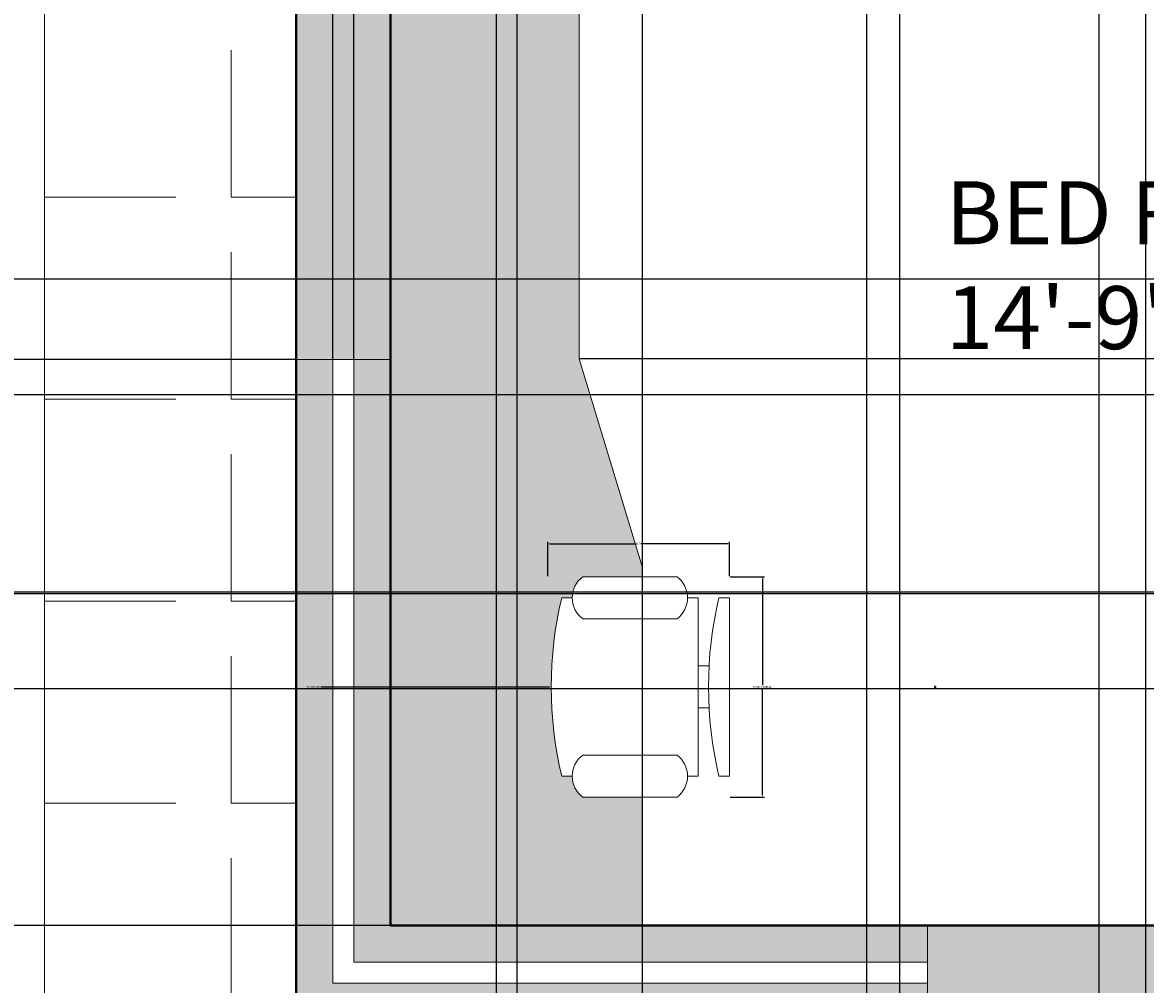
# Model space of a CAD drawing. Units: inches. Extents: x 818 to 1898, y 976 to 2364.
# Tile 21 of 96: x 1405 to 1512, y 1349 to 1441. Entities that reach past the tile are written whole.
import ezdxf

# ---------------------------------------------------------------- set-up
doc = ezdxf.new("R2010")
doc.units = ezdxf.units.IN
doc.header["$LTSCALE"] = 5
doc.header["$MEASUREMENT"] = 0
for name, color, linetype, lineweight in [('A-ANNO-DIMS', 2, 'Continuous', 18), ('A-AREA-IDEN', 7, 'Continuous', 18), ('A-FLOR-CASE', 8, 'Continuous', 18), ('A-FLOR-CASE-PATT', 33, 'Continuous', 9), ('A-FURN', 8, 'Continuous', 18), ('A-GLAZ', 4, 'Continuous', 18), ('A-WALL', 7, 'Continuous', 40), ('C-PKNG', 8, 'Continuous', 18), ('C-PKNG-PATT', 9, 'Continuous', 9)]:
    doc.layers.add(name, color=color, linetype=linetype, lineweight=lineweight)
doc.layers.add('A-GLAZ-PATT', color=141, linetype='Continuous', lineweight=9, true_color=0xadddf7)
doc.layers.add('A-WALL-PATT', color=251, linetype='Continuous', lineweight=13, true_color=0x636466)
doc.styles.get("Standard").update_dxf_attribs({"font": 'arial.ttf'})
doc.dimstyles.get("Standard").update_dxf_attribs({"dimtxt": 0.18, "dimasz": 0.18, "dimexe": 0.18, "dimexo": 0.0625, "dimgap": 0.09, "dimtad": 0, "dimtih": 1, "dimtoh": 1, "dimdec": 4, "dimzin": 0, "dimdsep": 46, "dimtxsty": 'Standard', "dimcen": 0.09, "dimadec": 0, "dimazin": 0, "dimtfac": 1, "dimtdec": 4, "dimtofl": 0, "dimtmove": 0, "dimatfit": 3, "dimfxl": 1, "dimtolj": 1, "dimtzin": 0, "dimarcsym": 0})
pattern_1 = [(0, (0, 0), (0, 19.25), [14, -5.25]), (90, (0, 0), (-19.25, 1e-15), [14, -5.25])]

# ---------------------------------------------------------------- blocks, each defined once
blk = doc.blocks.new('Chair - Desk')
for p, q in [((-8.5, 0), (-8.5, -1)), ((-8.5, 0), (8.5, 0)), ((8.5, 0), (8.5, -1)), ((-2, -3), (-2, -1.9355)), ((2, -1.9576), (2, -3)), ((-8.5, -3), (-8.5, -4)), ((-8.5, -3), (8.5, -3)), ((8.5, -3), (8.5, -4)), ((-10.5, -5), (-10.5, -14)), ((-6.5, -14), (-6.5, -5)), ((6.5, -5), (6.5, -14)), ((10.5, -14), (10.5, -5)), ((-8.5, -15), (-8.5, -16)), ((8.5, -15), (8.5, -16))]:
    blk.add_line(p, q)
for centre, radius, start, end in [((0, 34.625), 36.625, 256.5803, 283.4197), ((-8.5, -6.5), 2.5, 36.8699, 143.1301), ((8.5, -6.5), 2.5, 36.8699, 143.1301), ((-8.5, -12.5), 2.5, 216.8699, 323.1301), ((8.5, -12.5), 2.5, 216.8699, 323.1301), ((0, 19.625), 36.625, 256.5803, 283.4197)]:
    blk.add_arc(centre, radius, start, end)
blk = doc.blocks.new('*D54')
at = {"layer": 'A-ANNO-DIMS', "color": 0, "lineweight": -2, "ltscale": 5, "transparency": 16777216}
for p, q in [((1472.11, 1388.33), (1475.38, 1388.33)), ((1475.2, 1388.15), (1475.2, 1378.01)), ((1475.2, 1367.51), (1475.2, 1377.65)), ((1472.11, 1367.33), (1475.38, 1367.33))]:
    blk.add_line(p, q, dxfattribs=at)
at = {"layer": 'A-ANNO-DIMS', "color": 0, "ltscale": 5, "transparency": 16777216}
for points in [[(1475.17, 1388.15), (1475.23, 1388.15), (1475.2, 1388.33)], [(1475.17, 1367.51), (1475.23, 1367.51), (1475.2, 1367.33)]]:
    blk.add_solid(points, dxfattribs=at)
at = {"layer": 'Defpoints', "color": 0, "ltscale": 5, "transparency": 16777216}
for p in [(1472.05, 1388.33), (1472.05, 1367.33), (1475.2, 1367.33)]:
    blk.add_point(p, dxfattribs=at)
at = {"layer": 'A-ANNO-DIMS', "color": 0, "ltscale": 5, "transparency": 16777216, "insert": (1475.2, 1377.83), "char_height": 0.18, "attachment_point": 5}
blk.add_mtext('\\A1;DESK CHAIR 21', dxfattribs=at)
blk = doc.blocks.new('*D55')
at = {"layer": 'A-ANNO-DIMS', "color": 0, "lineweight": -2, "ltscale": 5, "transparency": 16777216}
for p, q in [((1454.71, 1388.39), (1454.71, 1391.66)), ((1454.89, 1391.48), (1463.17, 1391.48)), ((1471.87, 1391.48), (1463.59, 1391.48)), ((1472.05, 1388.39), (1472.05, 1391.66))]:
    blk.add_line(p, q, dxfattribs=at)
at = {"layer": 'A-ANNO-DIMS', "color": 0, "ltscale": 5, "transparency": 16777216}
for points in [[(1454.89, 1391.51), (1454.89, 1391.45), (1454.71, 1391.48)], [(1471.87, 1391.51), (1471.87, 1391.45), (1472.05, 1391.48)]]:
    blk.add_solid(points, dxfattribs=at)
at = {"layer": 'Defpoints', "color": 0, "ltscale": 5, "transparency": 16777216}
for p in [(1472.05, 1391.48), (1454.71, 1388.33), (1472.05, 1388.33)]:
    blk.add_point(p, dxfattribs=at)
at = {"layer": 'A-ANNO-DIMS', "color": 0, "ltscale": 5, "transparency": 16777216, "insert": (1463.38, 1391.48), "char_height": 0.18, "attachment_point": 5}
blk.add_mtext('\\A1;17', dxfattribs=at)
blk = doc.blocks.new('*D61')
at = {"layer": 'A-ANNO-DIMS', "color": 0, "lineweight": -2, "ltscale": 5, "transparency": 16777216}
for p, q in [((1071.73, 1203.03), (1071.73, 2363.87)), ((1430.73, 1203.03), (1430.73, 2363.87)), ((1071.91, 2363.69), (1250.94, 2363.69)), ((1430.55, 2363.69), (1251.51, 2363.69))]:
    blk.add_line(p, q, dxfattribs=at)
at = {"layer": 'A-ANNO-DIMS', "color": 0, "ltscale": 5, "transparency": 16777216}
for points in [[(1071.91, 2363.72), (1071.91, 2363.66), (1071.73, 2363.69)], [(1430.55, 2363.72), (1430.55, 2363.66), (1430.73, 2363.69)]]:
    blk.add_solid(points, dxfattribs=at)
at = {"layer": 'Defpoints', "color": 0, "ltscale": 5, "transparency": 16777216}
for p in [(1430.73, 2363.69), (1071.73, 1202.96), (1430.73, 1202.96)]:
    blk.add_point(p, dxfattribs=at)
at = {"layer": 'A-ANNO-DIMS', "color": 0, "ltscale": 5, "transparency": 16777216, "insert": (1251.23, 2363.69), "char_height": 0.18, "attachment_point": 5}
blk.add_mtext('\\A1;359', dxfattribs=at)
blk = doc.blocks.new('*D99')
at = {"layer": 'A-ANNO-DIMS', "color": 0, "lineweight": -2, "ltscale": 5, "transparency": 16777216}
for p, q in [((1391.88, 1071.12), (1391.88, 2363.87)), ((1449.82, 1071.12), (1449.82, 2363.87)), ((1392.06, 2363.69), (1420.45, 2363.69)), ((1449.64, 2363.69), (1421.24, 2363.69))]:
    blk.add_line(p, q, dxfattribs=at)
at = {"layer": 'A-ANNO-DIMS', "color": 0, "ltscale": 5, "transparency": 16777216}
for points in [[(1392.06, 2363.72), (1392.06, 2363.66), (1391.88, 2363.69)], [(1449.64, 2363.72), (1449.64, 2363.66), (1449.82, 2363.69)]]:
    blk.add_solid(points, dxfattribs=at)
at = {"layer": 'Defpoints', "color": 0, "ltscale": 5, "transparency": 16777216}
for p in [(1449.82, 2363.69), (1391.88, 1071.06), (1449.82, 1071.06)]:
    blk.add_point(p, dxfattribs=at)
at = {"layer": 'A-ANNO-DIMS', "color": 0, "ltscale": 5, "transparency": 16777216, "insert": (1420.85, 2363.69), "char_height": 0.18, "attachment_point": 5}
blk.add_mtext('\\A1;57.94', dxfattribs=at)
blk = doc.blocks.new('*D100')
at = {"layer": 'A-ANNO-DIMS', "color": 0, "lineweight": -2, "ltscale": 5, "transparency": 16777216}
for p, q in [((1449.82, 1071.12), (1449.82, 2363.87)), ((1507.3, 1071.12), (1507.3, 2363.87)), ((1450, 2363.69), (1478.17, 2363.69)), ((1507.12, 2363.69), (1478.95, 2363.69))]:
    blk.add_line(p, q, dxfattribs=at)
at = {"layer": 'A-ANNO-DIMS', "color": 0, "ltscale": 5, "transparency": 16777216}
for points in [[(1450, 2363.72), (1450, 2363.66), (1449.82, 2363.69)], [(1507.12, 2363.72), (1507.12, 2363.66), (1507.3, 2363.69)]]:
    blk.add_solid(points, dxfattribs=at)
at = {"layer": 'Defpoints', "color": 0, "ltscale": 5, "transparency": 16777216}
for p in [(1507.3, 2363.69), (1449.82, 1071.06), (1507.3, 1071.06)]:
    blk.add_point(p, dxfattribs=at)
at = {"layer": 'A-ANNO-DIMS', "color": 0, "ltscale": 5, "transparency": 16777216, "insert": (1478.56, 2363.69), "char_height": 0.18, "attachment_point": 5}
blk.add_mtext('\\A1;57.48', dxfattribs=at)
blk = doc.blocks.new('*D101')
at = {"layer": 'A-ANNO-DIMS', "color": 0, "lineweight": -2, "ltscale": 5, "transparency": 16777216}
for p, q in [((1507.3, 1071.12), (1507.3, 2363.87)), ((1565.48, 1071.12), (1565.48, 2363.87)), ((1507.48, 2363.69), (1536, 2363.69)), ((1565.3, 2363.69), (1536.78, 2363.69))]:
    blk.add_line(p, q, dxfattribs=at)
at = {"layer": 'A-ANNO-DIMS', "color": 0, "ltscale": 5, "transparency": 16777216}
for points in [[(1507.48, 2363.72), (1507.48, 2363.66), (1507.3, 2363.69)], [(1565.3, 2363.72), (1565.3, 2363.66), (1565.48, 2363.69)]]:
    blk.add_solid(points, dxfattribs=at)
at = {"layer": 'Defpoints', "color": 0, "ltscale": 5, "transparency": 16777216}
for p in [(1565.48, 2363.69), (1507.3, 1071.06), (1565.48, 1071.06)]:
    blk.add_point(p, dxfattribs=at)
at = {"layer": 'A-ANNO-DIMS', "color": 0, "ltscale": 5, "transparency": 16777216, "insert": (1536.39, 2363.69), "char_height": 0.18, "attachment_point": 5}
blk.add_mtext('\\A1;58.19', dxfattribs=at)
blk = doc.blocks.new('*D112')
at = {"layer": 'A-ANNO-DIMS', "color": 0, "lineweight": -2, "ltscale": 5, "transparency": 16777216}
for p, q in [((1135.27, 1405.71), (1897.92, 1405.71)), ((1897.74, 1405.53), (1897.74, 1396.48)), ((1897.74, 1387.07), (1897.74, 1396.12)), ((1135.27, 1386.89), (1897.92, 1386.89))]:
    blk.add_line(p, q, dxfattribs=at)
at = {"layer": 'A-ANNO-DIMS', "color": 0, "ltscale": 5, "transparency": 16777216}
for points in [[(1897.71, 1405.53), (1897.77, 1405.53), (1897.74, 1405.71)], [(1897.71, 1387.07), (1897.77, 1387.07), (1897.74, 1386.89)]]:
    blk.add_solid(points, dxfattribs=at)
at = {"layer": 'Defpoints', "color": 0, "ltscale": 5, "transparency": 16777216}
for p in [(1135.21, 1405.71), (1135.21, 1386.89), (1897.74, 1386.89)]:
    blk.add_point(p, dxfattribs=at)
at = {"layer": 'A-ANNO-DIMS', "color": 0, "ltscale": 5, "transparency": 16777216, "insert": (1897.74, 1396.3), "char_height": 0.18, "attachment_point": 5}
blk.add_mtext('\\A1;18.824', dxfattribs=at)
blk = doc.blocks.new('*D115')
at = {"layer": 'A-ANNO-DIMS', "color": 0, "lineweight": -2, "ltscale": 5, "transparency": 16777216}
for p, q in [((1766.29, 1377.66), (818.03, 1377.66)), ((818.21, 1377.48), (818.21, 1338.26)), ((818.21, 1298.68), (818.21, 1337.9)), ((1766.29, 1298.5), (818.03, 1298.5))]:
    blk.add_line(p, q, dxfattribs=at)
at = {"layer": 'A-ANNO-DIMS', "color": 0, "ltscale": 5, "transparency": 16777216}
for points in [[(818.18, 1377.48), (818.24, 1377.48), (818.21, 1377.66)], [(818.18, 1298.68), (818.24, 1298.68), (818.21, 1298.5)]]:
    blk.add_solid(points, dxfattribs=at)
at = {"layer": 'Defpoints', "color": 0, "ltscale": 5, "transparency": 16777216}
for p in [(818.21, 1377.66), (1766.35, 1377.66), (1766.35, 1298.5)]:
    blk.add_point(p, dxfattribs=at)
at = {"layer": 'A-ANNO-DIMS', "color": 0, "ltscale": 5, "transparency": 16777216, "insert": (818.21, 1338.08), "char_height": 0.18, "attachment_point": 5}
blk.add_mtext('\\A1;79.15', dxfattribs=at)
blk = doc.blocks.new('*D116')
at = {"layer": 'A-ANNO-DIMS', "color": 0, "lineweight": -2, "ltscale": 5, "transparency": 16777216}
for p, q in [((1766.29, 1456.81), (818.03, 1456.81)), ((818.21, 1456.63), (818.21, 1417.41)), ((818.21, 1377.84), (818.21, 1417.05)), ((1766.29, 1377.66), (818.03, 1377.66))]:
    blk.add_line(p, q, dxfattribs=at)
at = {"layer": 'A-ANNO-DIMS', "color": 0, "ltscale": 5, "transparency": 16777216}
for points in [[(818.18, 1456.63), (818.24, 1456.63), (818.21, 1456.81)], [(818.18, 1377.84), (818.24, 1377.84), (818.21, 1377.66)]]:
    blk.add_solid(points, dxfattribs=at)
at = {"layer": 'Defpoints', "color": 0, "ltscale": 5, "transparency": 16777216}
for p in [(818.21, 1456.81), (1766.35, 1456.81), (1766.35, 1377.66)]:
    blk.add_point(p, dxfattribs=at)
at = {"layer": 'A-ANNO-DIMS', "color": 0, "ltscale": 5, "transparency": 16777216, "insert": (818.21, 1417.23), "char_height": 0.18, "attachment_point": 5}
blk.add_mtext('\\A1;79.15', dxfattribs=at)
blk = doc.blocks.new('*D159')
at = {"layer": 'A-ANNO-DIMS', "color": 0, "lineweight": -2, "ltscale": 5, "transparency": 16777216}
for p, q in [((1206.73, 1687.02), (1206.73, 975.66)), ((1463.73, 1687.02), (1463.73, 975.66)), ((1206.91, 975.84), (1334.93, 975.84)), ((1463.55, 975.84), (1335.52, 975.84))]:
    blk.add_line(p, q, dxfattribs=at)
at = {"layer": 'A-ANNO-DIMS', "color": 0, "ltscale": 5, "transparency": 16777216}
for points in [[(1206.91, 975.87), (1206.91, 975.81), (1206.73, 975.84)], [(1463.55, 975.87), (1463.55, 975.81), (1463.73, 975.84)]]:
    blk.add_solid(points, dxfattribs=at)
at = {"layer": 'Defpoints', "color": 0, "ltscale": 5, "transparency": 16777216}
for p in [(1206.73, 1687.08), (1463.73, 1687.08), (1463.73, 975.84)]:
    blk.add_point(p, dxfattribs=at)
at = {"layer": 'A-ANNO-DIMS', "color": 0, "ltscale": 5, "transparency": 16777216, "insert": (1335.23, 975.84), "char_height": 0.18, "attachment_point": 5}
blk.add_mtext('\\A1;257', dxfattribs=at)
blk = doc.blocks.new('*D160')
at = {"layer": 'A-ANNO-DIMS', "color": 0, "lineweight": -2, "ltscale": 5, "transparency": 16777216}
for p, q in [((1463.73, 1687.02), (1463.73, 975.66)), ((1511.73, 1687.02), (1511.73, 975.66)), ((1463.91, 975.84), (1487.5, 975.84)), ((1511.55, 975.84), (1487.95, 975.84))]:
    blk.add_line(p, q, dxfattribs=at)
at = {"layer": 'A-ANNO-DIMS', "color": 0, "ltscale": 5, "transparency": 16777216}
for points in [[(1463.91, 975.87), (1463.91, 975.81), (1463.73, 975.84)], [(1511.55, 975.87), (1511.55, 975.81), (1511.73, 975.84)]]:
    blk.add_solid(points, dxfattribs=at)
at = {"layer": 'Defpoints', "color": 0, "ltscale": 5, "transparency": 16777216}
for p in [(1463.73, 1687.08), (1511.73, 1687.08), (1511.73, 975.84)]:
    blk.add_point(p, dxfattribs=at)
at = {"layer": 'A-ANNO-DIMS', "color": 0, "ltscale": 5, "transparency": 16777216, "insert": (1487.73, 975.84), "char_height": 0.18, "attachment_point": 5}
blk.add_mtext('\\A1;48', dxfattribs=at)
blk = doc.blocks.new('*D167')
at = {"layer": 'A-ANNO-DIMS', "color": 0, "lineweight": -2, "ltscale": 5, "transparency": 16777216}
for p, q in [((1345.97, 1486.18), (1345.97, 975.66)), ((1430.73, 1486.18), (1430.73, 975.66)), ((1346.15, 975.84), (1387.95, 975.84)), ((1430.55, 975.84), (1388.74, 975.84))]:
    blk.add_line(p, q, dxfattribs=at)
at = {"layer": 'A-ANNO-DIMS', "color": 0, "ltscale": 5, "transparency": 16777216}
for points in [[(1346.15, 975.87), (1346.15, 975.81), (1345.97, 975.84)], [(1430.55, 975.87), (1430.55, 975.81), (1430.73, 975.84)]]:
    blk.add_solid(points, dxfattribs=at)
at = {"layer": 'Defpoints', "color": 0, "ltscale": 5, "transparency": 16777216}
for p in [(1345.97, 1486.24), (1430.73, 1486.24), (1430.73, 975.84)]:
    blk.add_point(p, dxfattribs=at)
at = {"layer": 'A-ANNO-DIMS', "color": 0, "ltscale": 5, "transparency": 16777216, "insert": (1388.35, 975.84), "char_height": 0.18, "attachment_point": 5}
blk.add_mtext('\\A1;84.76', dxfattribs=at)
blk = doc.blocks.new('*D171')
at = {"layer": 'A-ANNO-DIMS', "color": 0, "lineweight": -2, "ltscale": 5, "transparency": 16777216}
for p, q in [((1616.66, 1386.69), (818.03, 1386.69)), ((818.21, 1386.51), (818.21, 1371.06)), ((818.21, 1355.26), (818.21, 1370.7)), ((1616.66, 1355.08), (818.03, 1355.08))]:
    blk.add_line(p, q, dxfattribs=at)
at = {"layer": 'A-ANNO-DIMS', "color": 0, "ltscale": 5, "transparency": 16777216}
for points in [[(818.18, 1386.51), (818.24, 1386.51), (818.21, 1386.69)], [(818.18, 1355.26), (818.24, 1355.26), (818.21, 1355.08)]]:
    blk.add_solid(points, dxfattribs=at)
at = {"layer": 'Defpoints', "color": 0, "ltscale": 5, "transparency": 16777216}
for p in [(818.21, 1386.69), (1616.73, 1386.69), (1616.73, 1355.08)]:
    blk.add_point(p, dxfattribs=at)
at = {"layer": 'A-ANNO-DIMS', "color": 0, "ltscale": 5, "transparency": 16777216, "insert": (818.21, 1370.88), "char_height": 0.18, "attachment_point": 5}
blk.add_mtext('\\A1;31.61', dxfattribs=at)
blk = doc.blocks.new('*D172')
at = {"layer": 'A-ANNO-DIMS', "color": 0, "lineweight": -2, "ltscale": 5, "transparency": 16777216}
for p, q in [((1616.66, 1416.69), (818.03, 1416.69)), ((818.21, 1416.51), (818.21, 1401.87)), ((818.21, 1386.87), (818.21, 1401.5)), ((1616.66, 1386.69), (818.03, 1386.69))]:
    blk.add_line(p, q, dxfattribs=at)
at = {"layer": 'A-ANNO-DIMS', "color": 0, "ltscale": 5, "transparency": 16777216}
for points in [[(818.18, 1416.51), (818.24, 1416.51), (818.21, 1416.69)], [(818.18, 1386.87), (818.24, 1386.87), (818.21, 1386.69)]]:
    blk.add_solid(points, dxfattribs=at)
at = {"layer": 'Defpoints', "color": 0, "ltscale": 5, "transparency": 16777216}
for p in [(818.21, 1416.69), (1616.73, 1416.69), (1616.73, 1386.69)]:
    blk.add_point(p, dxfattribs=at)
at = {"layer": 'A-ANNO-DIMS', "color": 0, "ltscale": 5, "transparency": 16777216, "insert": (818.21, 1401.69), "char_height": 0.18, "attachment_point": 5}
blk.add_mtext('\\A1;30', dxfattribs=at)
blk = doc.blocks.new('*D182')
at = {"layer": 'A-ANNO-DIMS', "color": 0, "lineweight": -2, "ltscale": 5, "transparency": 16777216}
for p, q in [((1463.73, 1687.02), (1463.73, 975.66)), ((1559.73, 1687.02), (1559.73, 975.66)), ((1463.91, 975.84), (1511.51, 975.84)), ((1559.55, 975.84), (1511.94, 975.84))]:
    blk.add_line(p, q, dxfattribs=at)
at = {"layer": 'A-ANNO-DIMS', "color": 0, "ltscale": 5, "transparency": 16777216}
for points in [[(1463.91, 975.87), (1463.91, 975.81), (1463.73, 975.84)], [(1559.55, 975.87), (1559.55, 975.81), (1559.73, 975.84)]]:
    blk.add_solid(points, dxfattribs=at)
at = {"layer": 'Defpoints', "color": 0, "ltscale": 5, "transparency": 16777216}
for p in [(1463.73, 1687.08), (1559.73, 1687.08), (1559.73, 975.84)]:
    blk.add_point(p, dxfattribs=at)
at = {"layer": 'A-ANNO-DIMS', "color": 0, "ltscale": 5, "transparency": 16777216, "insert": (1511.73, 975.84), "char_height": 0.18, "attachment_point": 5}
blk.add_mtext('\\A1;96', dxfattribs=at)
blk = doc.blocks.new('*D190')
at = {"layer": 'A-ANNO-DIMS', "color": 0, "lineweight": -2, "ltscale": 5, "transparency": 16777216}
for p, q in [((1430.66, 1409.05), (818.03, 1409.05)), ((818.21, 1408.87), (818.21, 1377.75)), ((818.21, 1346.26), (818.21, 1377.38)), ((1430.66, 1346.08), (818.03, 1346.08))]:
    blk.add_line(p, q, dxfattribs=at)
at = {"layer": 'A-ANNO-DIMS', "color": 0, "ltscale": 5, "transparency": 16777216}
for points in [[(818.18, 1408.87), (818.24, 1408.87), (818.21, 1409.05)], [(818.18, 1346.26), (818.24, 1346.26), (818.21, 1346.08)]]:
    blk.add_solid(points, dxfattribs=at)
at = {"layer": 'Defpoints', "color": 0, "ltscale": 5, "transparency": 16777216}
for p in [(818.21, 1409.05), (1430.73, 1409.05), (1430.73, 1346.08)]:
    blk.add_point(p, dxfattribs=at)
at = {"layer": 'A-ANNO-DIMS', "color": 0, "ltscale": 5, "transparency": 16777216, "insert": (818.21, 1377.57), "char_height": 0.18, "attachment_point": 5}
blk.add_mtext('\\A1;62.97', dxfattribs=at)
blk = doc.blocks.new('*D191')
at = {"layer": 'A-ANNO-DIMS', "color": 0, "lineweight": -2, "ltscale": 5, "transparency": 16777216}
for p, q in [((1434.23, 1409.11), (1434.23, 2363.87)), ((1436.23, 1409.11), (1436.23, 2363.87)), ((1434.41, 2363.69), (1435.08, 2363.69)), ((1436.05, 2363.69), (1435.37, 2363.69))]:
    blk.add_line(p, q, dxfattribs=at)
at = {"layer": 'A-ANNO-DIMS', "color": 0, "ltscale": 5, "transparency": 16777216}
for points in [[(1434.41, 2363.72), (1434.41, 2363.66), (1434.23, 2363.69)], [(1436.05, 2363.72), (1436.05, 2363.66), (1436.23, 2363.69)]]:
    blk.add_solid(points, dxfattribs=at)
at = {"layer": 'Defpoints', "color": 0, "ltscale": 5, "transparency": 16777216}
for p in [(1436.23, 2363.69), (1434.23, 1409.05), (1436.23, 1409.05)]:
    blk.add_point(p, dxfattribs=at)
at = {"layer": 'A-ANNO-DIMS', "color": 0, "ltscale": 5, "transparency": 16777216, "insert": (1435.23, 2363.69), "char_height": 0.18, "attachment_point": 5}
blk.add_mtext('\\A1;2', dxfattribs=at)
blk = doc.blocks.new('*D197')
at = {"layer": 'A-ANNO-DIMS', "color": 0, "lineweight": -2, "ltscale": 5, "transparency": 16777216}
for p, q in [((1457.79, 1526.67), (1897.92, 1526.67)), ((1897.74, 1526.49), (1897.74, 1468.08)), ((1897.74, 1409.3), (1897.74, 1467.71)), ((1457.79, 1409.12), (1897.92, 1409.12))]:
    blk.add_line(p, q, dxfattribs=at)
at = {"layer": 'A-ANNO-DIMS', "color": 0, "ltscale": 5, "transparency": 16777216}
for points in [[(1897.71, 1526.49), (1897.77, 1526.49), (1897.74, 1526.67)], [(1897.71, 1409.3), (1897.77, 1409.3), (1897.74, 1409.12)]]:
    blk.add_solid(points, dxfattribs=at)
at = {"layer": 'Defpoints', "color": 0, "ltscale": 5, "transparency": 16777216}
for p in [(1457.73, 1526.67), (1897.74, 1526.67), (1457.73, 1409.12)]:
    blk.add_point(p, dxfattribs=at)
at = {"layer": 'A-ANNO-DIMS', "color": 0, "ltscale": 5, "transparency": 16777216, "insert": (1897.74, 1467.89), "char_height": 0.18, "attachment_point": 5}
blk.add_mtext('\\A1;117.55', dxfattribs=at)
blk = doc.blocks.new('*D198')
at = {"layer": 'A-ANNO-DIMS', "color": 0, "lineweight": -2, "ltscale": 5, "transparency": 16777216}
for p, q in [((1741.84, 1545.02), (1741.84, 975.66)), ((1430.73, 1346.02), (1430.73, 975.66)), ((1430.91, 975.84), (1585.91, 975.84)), ((1741.66, 975.84), (1586.66, 975.84))]:
    blk.add_line(p, q, dxfattribs=at)
at = {"layer": 'A-ANNO-DIMS', "color": 0, "ltscale": 5, "transparency": 16777216}
for points in [[(1430.91, 975.87), (1430.91, 975.81), (1430.73, 975.84)], [(1741.66, 975.87), (1741.66, 975.81), (1741.84, 975.84)]]:
    blk.add_solid(points, dxfattribs=at)
at = {"layer": 'Defpoints', "color": 0, "ltscale": 5, "transparency": 16777216}
for p in [(1741.84, 1545.08), (1430.73, 1346.08), (1741.84, 975.84)]:
    blk.add_point(p, dxfattribs=at)
at = {"layer": 'A-ANNO-DIMS', "color": 0, "ltscale": 5, "transparency": 16777216, "insert": (1586.28, 975.84), "char_height": 0.18, "attachment_point": 5}
blk.add_mtext('\\A1;311.1', dxfattribs=at)
blk = doc.blocks.new('*D214')
at = {"layer": 'A-ANNO-DIMS', "color": 0, "lineweight": -2, "ltscale": 5, "transparency": 16777216}
for p, q in [((1511.73, 1687.02), (1511.73, 975.66)), ((1714.73, 1687.02), (1714.73, 975.66)), ((1511.91, 975.84), (1612.93, 975.84)), ((1714.55, 975.84), (1613.52, 975.84))]:
    blk.add_line(p, q, dxfattribs=at)
at = {"layer": 'A-ANNO-DIMS', "color": 0, "ltscale": 5, "transparency": 16777216}
for points in [[(1511.91, 975.87), (1511.91, 975.81), (1511.73, 975.84)], [(1714.55, 975.87), (1714.55, 975.81), (1714.73, 975.84)]]:
    blk.add_solid(points, dxfattribs=at)
at = {"layer": 'Defpoints', "color": 0, "ltscale": 5, "transparency": 16777216}
for p in [(1511.73, 1687.08), (1714.73, 1687.08), (1714.73, 975.84)]:
    blk.add_point(p, dxfattribs=at)
at = {"layer": 'A-ANNO-DIMS', "color": 0, "ltscale": 5, "transparency": 16777216, "insert": (1613.23, 975.84), "char_height": 0.18, "attachment_point": 5}
blk.add_mtext('\\A1;203', dxfattribs=at)
blk = doc.blocks.new('*D242')
at = {"layer": 'A-ANNO-DIMS', "color": 0, "lineweight": -2, "ltscale": 5, "transparency": 16777216}
for p, q in [((1488.26, 1948.6), (1488.26, 975.66)), ((1513.23, 1948.6), (1513.23, 975.66)), ((1488.44, 975.84), (1500.35, 975.84)), ((1513.05, 975.84), (1501.14, 975.84))]:
    blk.add_line(p, q, dxfattribs=at)
at = {"layer": 'A-ANNO-DIMS', "color": 0, "ltscale": 5, "transparency": 16777216}
for points in [[(1488.44, 975.87), (1488.44, 975.81), (1488.26, 975.84)], [(1513.05, 975.87), (1513.05, 975.81), (1513.23, 975.84)]]:
    blk.add_solid(points, dxfattribs=at)
at = {"layer": 'Defpoints', "color": 0, "ltscale": 5, "transparency": 16777216}
for p in [(1488.26, 1948.66), (1513.23, 1948.66), (1513.23, 975.84)]:
    blk.add_point(p, dxfattribs=at)
at = {"layer": 'A-ANNO-DIMS', "color": 0, "ltscale": 5, "transparency": 16777216, "insert": (1500.74, 975.84), "char_height": 0.18, "attachment_point": 5}
blk.add_mtext('\\A1;24.97', dxfattribs=at)
blk = doc.blocks.new('*D243')
at = {"layer": 'A-ANNO-DIMS', "color": 0, "lineweight": -2, "ltscale": 5, "transparency": 16777216}
for p, q in [((1451.77, 2020.02), (1451.77, 975.66)), ((1590.73, 2020.02), (1590.73, 975.66)), ((1451.95, 975.84), (1520.79, 975.84)), ((1590.55, 975.84), (1521.7, 975.84))]:
    blk.add_line(p, q, dxfattribs=at)
at = {"layer": 'A-ANNO-DIMS', "color": 0, "ltscale": 5, "transparency": 16777216}
for points in [[(1451.95, 975.87), (1451.95, 975.81), (1451.77, 975.84)], [(1590.55, 975.87), (1590.55, 975.81), (1590.73, 975.84)]]:
    blk.add_solid(points, dxfattribs=at)
at = {"layer": 'Defpoints', "color": 0, "ltscale": 5, "transparency": 16777216}
for p in [(1451.77, 2020.08), (1590.73, 2020.08), (1590.73, 975.84)]:
    blk.add_point(p, dxfattribs=at)
at = {"layer": 'A-ANNO-DIMS', "color": 0, "ltscale": 5, "transparency": 16777216, "insert": (1521.25, 975.84), "char_height": 0.18, "attachment_point": 5}
blk.add_mtext('\\A1;138.96', dxfattribs=at)
blk = doc.blocks.new('*D253')
at = {"layer": 'A-ANNO-DIMS', "color": 0, "lineweight": -2, "ltscale": 5, "transparency": 16777216}
for p, q in [((1485.12, 2053.02), (1485.12, 975.66)), ((1538.52, 2053.02), (1538.52, 975.66)), ((1485.3, 975.84), (1511.42, 975.84)), ((1538.34, 975.84), (1512.21, 975.84))]:
    blk.add_line(p, q, dxfattribs=at)
at = {"layer": 'A-ANNO-DIMS', "color": 0, "ltscale": 5, "transparency": 16777216}
for points in [[(1485.3, 975.87), (1485.3, 975.81), (1485.12, 975.84)], [(1538.34, 975.87), (1538.34, 975.81), (1538.52, 975.84)]]:
    blk.add_solid(points, dxfattribs=at)
at = {"layer": 'Defpoints', "color": 0, "ltscale": 5, "transparency": 16777216}
for p in [(1485.12, 2053.08), (1538.52, 2053.08), (1538.52, 975.84)]:
    blk.add_point(p, dxfattribs=at)
at = {"layer": 'A-ANNO-DIMS', "color": 0, "ltscale": 5, "transparency": 16777216, "insert": (1511.82, 975.84), "char_height": 0.18, "attachment_point": 5}
blk.add_mtext('\\A1;53.39', dxfattribs=at)
blk = doc.blocks.new('*D294')
at = {"layer": 'A-ANNO-DIMS', "color": 0, "lineweight": -2, "ltscale": 5, "transparency": 16777216}
for p, q in [((1433.07, 1377.83), (1454.87, 1377.83)), ((1491.58, 1377.83), (1491.76, 1377.83)), ((1491.67, 1377.74), (1491.67, 1377.92))]:
    blk.add_line(p, q, dxfattribs=at)
at = {"layer": 'A-ANNO-DIMS', "color": 0, "ltscale": 5, "transparency": 16777216}
blk.add_solid([(1454.87, 1377.86), (1454.87, 1377.8), (1455.05, 1377.83)], dxfattribs=at)
at = {"layer": 'Defpoints', "color": 0, "ltscale": 5, "transparency": 16777216}
for p in [(1455.05, 1377.83), (1491.67, 1377.83)]:
    blk.add_point(p, dxfattribs=at)
at = {"layer": 'A-ANNO-DIMS', "color": 0, "ltscale": 5, "transparency": 16777216, "insert": (1432.33, 1377.83), "char_height": 0.18, "attachment_point": 5}
blk.add_mtext('\\A1;2X R36.625', dxfattribs=at)

msp = doc.modelspace()

# ---------------------------------------------------------------- hatches: boundary and pattern name
at = {"layer": 'A-FLOR-CASE-PATT', "ltscale": 5}
h = msp.add_hatch(color=256, dxfattribs=at)
h.dxf.hatch_style = 1
h.paths.add_polyline_path([(1705.7252, 1941.0782), (1681.7252, 1941.0782), (1681.7252, 1900.0782), (1599.7252, 1900.0782), (1599.7252, 1876.0782), (1705.7252, 1876.0782)])
h.paths.add_polyline_path([(1457.7251, 1409.1177), (1457.7251, 1526.6712), (1439.7252, 1526.6712), (1439.7252, 1457.5313), (1446.3307, 1457.5313), (1446.3307, 1468.9514), (1446.8307, 1470.665), (1446.8307, 1469.665), (1446.8307, 1468.9514), (1446.8307, 1456.8361), (1446.8307, 1444.7258), (1446.8307, 1443.3338), (1446.3307, 1444.7258), (1446.3307, 1456.8361), (1439.7252, 1456.8361), (1439.7252, 1355.0782), (1463.7251, 1355.0782), (1463.7251, 1367.3287), (1458.0475, 1367.3287, -0.23606798), (1457.0475, 1369.3287), (1456.0475, 1369.3287, -0.11764706), (1456.0475, 1386.3287), (1457.0475, 1386.3287, -0.23606798), (1458.0475, 1388.3287), (1463.7251, 1388.3287), (1463.7251, 1389.3211)])
h.paths.add_polyline_path([(1341.2593, 1534.0782), (1246.9377, 1534.0782), (1246.9377, 1510.0782), (1341.2593, 1510.0782)])
h.paths.add_polyline_path([(1288.8272, 1519.927), (1289.8272, 1519.927), (1290.5408, 1519.927), (1302.6561, 1519.927), (1314.7664, 1519.927), (1316.1584, 1519.927), (1314.7664, 1519.427), (1302.6561, 1519.427), (1302.6561, 1512.8214), (1301.9609, 1512.8214), (1301.9609, 1519.427), (1290.5408, 1519.427)], flags=16)
h.paths.add_polyline_path([(1377.7791, 1867.0782), (1344.5531, 1867.0782), (1344.5531, 1860.4726), (1355.9731, 1860.4726), (1357.6867, 1859.9726), (1356.6867, 1859.9726), (1355.9731, 1859.9726), (1343.8579, 1859.9726), (1331.7475, 1859.9726), (1330.3556, 1859.9726), (1331.7475, 1860.4726), (1343.8579, 1860.4726), (1343.8579, 1867.0782), (1311.3271, 1867.0782), (1311.3271, 1853.7496), (1377.7791, 1853.7496)])
h.paths.add_polyline_path([(1301.148, 1610.7299, -0.46196039), (1314.4882, 1599.3725, -0.19222541), (1311.3254, 1591.4497, 0.54791519), (1336.8832, 1607.7707, 0.92061359)])
h.paths.add_polyline_path([(1370.719, 1780.5695, 1), (1332.478, 1780.5695, 1)])
h.paths.add_polyline_path([(1705.7252, 1463.0782), (1681.7252, 1463.0782), (1681.7252, 1379.0782), (1622.7252, 1379.0782), (1622.7252, 1355.0782), (1705.7252, 1355.0782)])
h.paths.add_polyline_path([(1658.1052, 1359.2188), (1658.1786, 1359.2188), (1658.1786, 1373.8763), (1658.1052, 1373.9202)], flags=16)
h.paths.add_polyline_path([(1686.9271, 1409.9311), (1686.8832, 1409.8578), (1701.5845, 1409.8578), (1701.5845, 1409.9311)], flags=16)
h.paths.add_polyline_path([(1637.1266, 1359.2188), (1637.2, 1359.2188), (1637.2, 1373.8763), (1637.1266, 1373.9202)], flags=16)
at = {"layer": 'A-GLAZ-PATT', "ltscale": 5}
h = msp.add_hatch(color=256, dxfattribs=at)
h.dxf.hatch_style = 1
h.paths.add_polyline_path([(1283.8183, 1504.5782), (1206.7251, 1504.5782), (1206.7251, 1501.0782), (1283.8183, 1501.0782)])
h.paths.add_polyline_path([(1283.8183, 1510.0782), (1206.7251, 1510.0782), (1206.7251, 1506.5782), (1283.8183, 1506.5782)])
h.paths.add_polyline_path([(1490.9163, 1355.0782), (1439.7252, 1355.0782), (1439.7252, 1409.0522), (1436.2251, 1409.0522), (1436.2251, 1351.5782), (1490.9163, 1351.5782)])
h.paths.add_polyline_path([(1434.2251, 1409.0522), (1430.7251, 1409.0522), (1430.7251, 1346.0782), (1435.0799, 1346.0782), (1435.0731, 1346.1152), (1435.1501, 1346.0782), (1490.9163, 1346.0782), (1490.9163, 1349.5782), (1434.2251, 1349.5782)])
h.paths.add_polyline_path([(1714.7251, 1545.0782), (1711.2252, 1545.0782), (1711.2252, 1521.0782), (1714.7251, 1521.0782)])
h.paths.add_polyline_path([(1709.2252, 1545.0782), (1705.7252, 1545.0782), (1705.7252, 1521.0782), (1709.2252, 1521.0782)])
h.paths.add_polyline_path([(1714.7251, 1687.0782), (1711.2252, 1687.0782), (1711.2252, 1649.9029), (1714.7251, 1649.9029)])
h.paths.add_polyline_path([(1709.2252, 1687.0782), (1705.7252, 1687.0782), (1705.7252, 1649.9029), (1709.2252, 1649.9029)])
h.paths.add_polyline_path([(1709.2252, 1745.5584), (1705.7252, 1745.5584), (1705.7252, 1717.3178), (1709.2252, 1717.3178)])
h.paths.add_polyline_path([(1714.7251, 1745.5584), (1711.2252, 1745.5584), (1711.2252, 1717.3178), (1714.7251, 1717.3178)])
h.paths.add_polyline_path([(1714.7251, 2014.5114), (1711.2252, 2014.5114), (1711.2252, 1962.0338), (1714.7251, 1962.0338)])
h.paths.add_polyline_path([(1709.2252, 2014.5114), (1705.7252, 2014.5114), (1705.7252, 1962.0338), (1709.2252, 1962.0338)])
h.paths.add_polyline_path([(1538.5155, 2047.5782), (1485.1216, 2047.5782), (1485.1216, 2044.0782), (1538.5155, 2044.0782)])
h.paths.add_polyline_path([(1538.5155, 2053.0782), (1485.1216, 2053.0782), (1485.1216, 2049.5782), (1538.5155, 2049.5782)])
h.paths.add_polyline_path([(1388.0315, 2047.5782), (1330.305, 2047.5782), (1330.305, 2044.0782), (1388.0315, 2044.0782)])
h.paths.add_polyline_path([(1388.0315, 2053.0782), (1330.305, 2053.0782), (1330.305, 2049.5782), (1388.0315, 2049.5782)])
h.paths.add_polyline_path([(1262.2252, 2019.2871), (1258.7252, 2019.2871), (1258.7252, 1928.9218), (1262.2252, 1928.9218)])
h.paths.add_polyline_path([(1267.7252, 2019.2871), (1264.2252, 2019.2871), (1264.2252, 1928.9218), (1267.7252, 1928.9218)])
h.paths.add_polyline_path([(1262.2252, 1862.9652), (1258.7252, 1862.9652), (1258.7252, 1814.9652), (1262.2252, 1814.9652)])
h.paths.add_polyline_path([(1267.7252, 1862.9652), (1264.2252, 1862.9652), (1264.2252, 1814.9652), (1267.7252, 1814.9652)])
h.paths.add_polyline_path([(1262.2252, 1755.3321), (1258.7252, 1755.3321), (1258.7252, 1707.3321), (1262.2252, 1707.3321)])
h.paths.add_polyline_path([(1267.7252, 1755.3321), (1264.2252, 1755.3321), (1264.2252, 1707.3321), (1267.7252, 1707.3321)])
h.paths.add_polyline_path([(1251.9333, 1692.5782), (1206.7251, 1692.5782), (1206.7251, 1687.0782), (1251.9333, 1687.0782)])
h.paths.add_polyline_path([(1251.9333, 1700.0782), (1206.7251, 1700.0782), (1206.7251, 1694.5782), (1251.9333, 1694.5782)])
at = {"layer": 'A-WALL-PATT', "ltscale": 5}
h = msp.add_hatch(color=256, dxfattribs=at)
h.dxf.hatch_style = 1
h.paths.add_polyline_path([(1206.7251, 1687.0782), (1206.7251, 1700.0782), (1197.7252, 1700.0782), (1197.7252, 1501.0782), (1206.7251, 1501.0782), (1206.7251, 1510.0782)])
h.paths.add_polyline_path([(1197.7252, 1590.7585), (1173.7252, 1590.7585), (1173.7252, 1586.7585), (1197.7252, 1586.7585)])
h.paths.add_polyline_path([(1197.7252, 1534.6024), (1173.7252, 1534.6024), (1173.7252, 1530.6024), (1197.7252, 1530.6024)])
h.paths.add_polyline_path([(1365.1463, 1510.0782), (1283.8183, 1510.0782), (1283.8183, 1501.0782), (1365.1463, 1501.0782)])
h.paths.add_polyline_path([(1439.7252, 1591.0782), (1441.7252, 1591.0782), (1441.7252, 1600.0782), (1430.7251, 1600.0782), (1430.7251, 1510.0782), (1406.7252, 1510.0782), (1401.1463, 1510.0782), (1401.1463, 1501.0782), (1430.7251, 1501.0782), (1430.7251, 1486.2383), (1430.7251, 1409.0522), (1439.7252, 1409.0522)])
h = msp.add_hatch(color=256, dxfattribs=at)
h.dxf.hatch_style = 1
h.paths.add_polyline_path([(1714.7251, 1521.0782), (1705.7252, 1521.0782), (1705.7252, 1467.0782), (1654.7252, 1467.0782), (1654.7252, 1463.0782), (1705.7252, 1463.0782), (1705.7252, 1355.0782), (1622.7252, 1355.0782), (1622.7252, 1379.0782), (1622.7252, 1386.6857), (1616.7251, 1386.6857), (1616.7251, 1355.0782), (1490.9163, 1355.0782), (1490.9163, 1346.0782), (1544.7605, 1346.0782), (1544.6132, 1346.8783), (1544.6729, 1346.84), (1544.6299, 1346.7874), (1544.7605, 1346.0782), (1555.1299, 1346.0782), (1555.1299, 1341.5528), (1556.1599, 1340.8639), (1556.5281, 1338.8654), (1660.3141, 1338.8654), (1660.3141, 1346.0782), (1705.7252, 1346.0782), (1705.7252, 1345.0768), (1705.8704, 1344.58), (1705.7252, 1344.3933), (1705.7252, 1334.9904), (1705.8704, 1334.4936), (1705.7252, 1334.3068), (1705.7252, 1316.2253), (1707.3573, 1316.7694), (1707.3847, 1316.8046), (1707.3807, 1316.7771), (1705.7252, 1316.2253), (1705.7252, 1314.1392), (1705.7252, 1312.0957), (1705.8703, 1312.0739), (1705.7252, 1311.8873), (1705.7252, 1310.7121), (1706.5603, 1307.9282), (1707.8887, 1307.1831), (1714.7251, 1307.1831), (1714.7251, 1346.0782)])
at = {"layer": 'C-PKNG-PATT', "ltscale": 5}
h = msp.add_hatch(dxfattribs=at)
h.set_pattern_fill('ANGLE', color=256, scale=70)
h.set_pattern_definition(pattern_1)
h.paths.add_polyline_path([(1430.7251, 1211.9642), (1430.7251, 1486.2383), (1406.7252, 1486.2383), (1406.7252, 1235.9642), (1116.1882, 1235.9642), (1116.1882, 1485.2035), (1345.9651, 1485.2035), (1345.9651, 1501.0782), (1206.7251, 1501.0782), (1197.7252, 1501.0782), (1083.7252, 1501.0782), (1083.7252, 1485.2035), (1083.7252, 1211.9642)])
h = msp.add_hatch(dxfattribs=at)
h.set_pattern_fill('ANGLE', color=256, scale=70)
h.set_pattern_definition(pattern_1)
h.paths.add_polyline_path([(1116.1882, 1485.2035), (1345.9651, 1485.2035), (1345.9651, 1501.0782), (1206.7251, 1501.0782), (1197.7252, 1501.0782), (1083.7252, 1501.0782), (1083.7252, 1485.2035), (1083.7252, 1211.9642), (1430.7251, 1211.9642), (1430.7251, 1271.1621), (1430.7251, 1290.0782), (1430.7251, 1346.0782), (1430.7251, 1486.2383), (1406.7252, 1486.2383), (1406.7252, 1235.9642), (1116.1882, 1235.9642)])

# ---------------------------------------------------------------- linework, layer by layer
at = {"layer": 'A-FLOR-CASE'}
for p, q in [((1457.7251, 1526.6712), (1457.7251, 1409.1177)), ((1457.7251, 1409.1177), (1463.7251, 1389.3211)), ((1463.7251, 1389.3211), (1463.7251, 1355.0782))]:
    msp.add_line(p, q, dxfattribs=at)
at = {"layer": 'A-GLAZ'}
for p, q in [((1439.7252, 1409.0522), (1430.7251, 1409.0522)), ((1490.9163, 1355.0782), (1490.9163, 1346.0782))]:
    msp.add_line(p, q, dxfattribs=at)
for points in [[(1434.2251, 1409.0522), (1434.2251, 1349.5782), (1490.9163, 1349.5782)], [(1436.2251, 1409.0522), (1436.2251, 1351.5782), (1490.9163, 1351.5782)]]:
    msp.add_lwpolyline(points, dxfattribs=at)
at = {"layer": 'A-WALL'}
for p, q in [((1439.7252, 1591.0782), (1439.7252, 1355.0782)), ((1430.7251, 1501.0782), (1430.7251, 1346.0782)), ((1439.7252, 1355.0782), (1616.7251, 1355.0782))]:
    msp.add_line(p, q, dxfattribs=at)
at = {"layer": 'C-PKNG'}
msp.add_line((1406.7252, 1486.2383), (1406.7252, 1235.9642), dxfattribs=at)

# ---------------------------------------------------------------- block references
at = {"layer": 'A-FURN', "rotation": 270}
msp.add_blockref('Chair - Desk', (1472.0475, 1377.8287), dxfattribs=at)

# ---------------------------------------------------------------- texts
at = {"layer": 'A-AREA-IDEN', "ltscale": 5, "insert": (1492.6678, 1426.0314), "char_height": 6, "attachment_point": 1}
msp.add_mtext_dynamic_manual_height_columns('BED ROOM-1\\P14\'-9" X 19\'-8"', width=118.992422, gutter_width=1, heights=[0], dxfattribs=at)

# ---------------------------------------------------------------- dimensions: what is measured, and where the dimension line sits
at = {"layer": 'A-ANNO-DIMS', "ltscale": 5}
for base, p1, p2, override, picture, middle in [((1430.7251, 2363.6929), (1071.7251, 1202.9642), (1430.7251, 1202.9642), {"dimdec": 0, "dimlfac": 1, "dimrnd": 0, "dimzin": 0, "dimdsep": 46, "dimlunit": 2}, '*D61', (1251.2251, 2363.6929)), ((1449.8196, 2363.6929), (1391.8757, 1071.0552), (1449.8196, 1071.0552), {"dimdec": 2, "dimlfac": 1, "dimrnd": 0, "dimzin": 0, "dimdsep": 46, "dimlunit": 2}, '*D99', (1420.8477, 2363.6929)), ((1436.2251, 2363.6929), (1434.2251, 1409.0522), (1436.2251, 1409.0522), {"dimdec": 0, "dimlfac": 1, "dimrnd": 0, "dimzin": 0, "dimdsep": 46, "dimlunit": 2}, '*D191', (1435.2251, 2363.6929)), ((1507.2982, 2363.6929), (1449.8196, 1071.0552), (1507.2982, 1071.0552), {"dimdec": 2, "dimlfac": 1, "dimrnd": 0, "dimzin": 0, "dimdsep": 46, "dimlunit": 2}, '*D100', (1478.5589, 2363.6929)), ((1565.4835, 2363.6929), (1507.2982, 1071.0552), (1565.4835, 1071.0552), {"dimdec": 2, "dimlfac": 1, "dimrnd": 0, "dimzin": 0, "dimdsep": 46, "dimlunit": 2}, '*D101', (1536.3908, 2363.6929)), ((1538.5155, 975.8433), (1485.1216, 2053.0782), (1538.5155, 2053.0782), {"dimdec": 2, "dimlfac": 1, "dimrnd": 0, "dimzin": 0, "dimdsep": 46, "dimlunit": 2}, '*D253', (1511.8185, 975.8433)), ((1590.7251, 975.8433), (1451.7698, 2020.0782), (1590.7251, 2020.0782), {"dimdec": 2, "dimlfac": 1, "dimrnd": 0, "dimzin": 0, "dimdsep": 46, "dimlunit": 2}, '*D243', (1521.2475, 975.8433)), ((1513.2306, 975.8433), (1488.2586, 1948.6602), (1513.2306, 1948.6602), {"dimdec": 2, "dimlfac": 1, "dimrnd": 0, "dimzin": 0, "dimdsep": 46, "dimlunit": 2}, '*D242', (1500.7446, 975.8433)), ((1463.7251, 975.8433), (1206.7251, 1687.0782), (1463.7251, 1687.0782), {"dimdec": 0, "dimlfac": 1, "dimrnd": 0, "dimzin": 0, "dimdsep": 46, "dimlunit": 2}, '*D159', (1335.2251, 975.8433)), ((1511.7251, 975.8433), (1463.7251, 1687.0782), (1511.7251, 1687.0782), {"dimdec": 0, "dimlfac": 1, "dimrnd": 0, "dimzin": 0, "dimdsep": 46, "dimlunit": 2}, '*D160', (1487.7251, 975.8433)), ((1559.7251, 975.8433), (1463.7251, 1687.0782), (1559.7251, 1687.0782), {"dimdec": 0, "dimlfac": 1, "dimrnd": 0, "dimzin": 0, "dimdsep": 46, "dimlunit": 2}, '*D182', (1511.7251, 975.8433)), ((1714.7251, 975.8433), (1511.7251, 1687.0782), (1714.7251, 1687.0782), {"dimdec": 0, "dimlfac": 1, "dimrnd": 0, "dimzin": 0, "dimdsep": 46, "dimlunit": 2}, '*D214', (1613.2251, 975.8433)), ((1741.8409, 975.8433), (1430.7251, 1346.0782), (1741.8409, 1545.0782), {"dimdec": 1, "dimlfac": 1, "dimrnd": 0, "dimzin": 0, "dimdsep": 46, "dimlunit": 2}, '*D198', (1586.283, 975.8433)), ((1430.7251, 975.8433), (1345.9651, 1486.2383), (1430.7251, 1486.2383), {"dimdec": 2, "dimlfac": 1, "dimrnd": 0, "dimzin": 0, "dimdsep": 46, "dimlunit": 2}, '*D167', (1388.3451, 975.8433)), ((1472.0475, 1391.4787), (1454.7142, 1388.3287), (1472.0475, 1388.3287), {"dimdec": 0, "dimlfac": 1, "dimrnd": 0, "dimzin": 0, "dimdsep": 46, "dimlunit": 2}, '*D55', (1463.3808, 1391.4787))]:
    dim = msp.add_linear_dim(base=base, p1=p1, p2=p2, dimstyle='Standard', override=override, dxfattribs=at)
    dim.commit()
    dim.dimension.update_dxf_attribs({"geometry": picture, "text_midpoint": middle})
for base, p1, p2, override, picture, middle in [((1897.736, 1526.6712), (1457.7251, 1409.1177), (1457.7251, 1526.6712), {"dimdec": 2, "dimlfac": 1, "dimrnd": 0, "dimzin": 0, "dimdsep": 46, "dimlunit": 2}, '*D197', (1897.736, 1467.8945)), ((818.2059, 1456.8088), (1766.3524, 1377.6564), (1766.3524, 1456.8088), {"dimdec": 2, "dimlfac": 1, "dimrnd": 0, "dimzin": 0, "dimdsep": 46, "dimlunit": 2}, '*D116', (818.2059, 1417.2326)), ((818.2059, 1416.6857), (1616.7251, 1386.6857), (1616.7251, 1416.6857), {"dimdec": 0, "dimlfac": 1, "dimrnd": 0, "dimzin": 0, "dimdsep": 46, "dimlunit": 2}, '*D172', (818.2059, 1401.6857)), ((818.2059, 1409.0522), (1430.7251, 1346.0782), (1430.7251, 1409.0522), {"dimdec": 2, "dimlfac": 1, "dimrnd": 0, "dimzin": 0, "dimdsep": 46, "dimlunit": 2}, '*D190', (818.2059, 1377.5652)), ((1897.736, 1386.8851), (1135.2058, 1405.7088), (1135.2058, 1386.8851), {"dimdec": 3, "dimlfac": 1, "dimrnd": 0, "dimzin": 0, "dimdsep": 46, "dimlunit": 2}, '*D112', (1897.736, 1396.297)), ((818.2059, 1386.6857), (1616.7251, 1355.0782), (1616.7251, 1386.6857), {"dimdec": 2, "dimlfac": 1, "dimrnd": 0, "dimzin": 0, "dimdsep": 46, "dimlunit": 2}, '*D171', (818.2059, 1370.882)), ((818.2059, 1377.6564), (1766.3524, 1298.5041), (1766.3524, 1377.6564), {"dimdec": 2, "dimlfac": 1, "dimrnd": 0, "dimzin": 0, "dimdsep": 46, "dimlunit": 2}, '*D115', (818.2059, 1338.0803))]:
    dim = msp.add_linear_dim(base=base, p1=p1, p2=p2, angle=90, dimstyle='Standard', override=override, dxfattribs=at)
    dim.commit()
    dim.dimension.update_dxf_attribs({"geometry": picture, "text_midpoint": middle})
dim = msp.add_linear_dim(base=(1475.1975, 1367.3287), p1=(1472.0475, 1388.3287), p2=(1472.0475, 1367.3287), angle=270, text='DESK CHAIR <>', dimstyle='Standard', override={"dimdec": 0, "dimlfac": 1, "dimrnd": 0, "dimzin": 0, "dimdsep": 46, "dimlunit": 2}, dxfattribs=at)
dim.commit()
dim.dimension.update_dxf_attribs({"geometry": '*D54', "text_midpoint": (1475.1975, 1377.8287)})
dim = msp.add_radius_dim(center=(1491.6725, 1377.8287), mpoint=(1455.0475, 1377.829), text='2X <>', dimstyle='Standard', override={"dimdec": 3, "dimlfac": 1, "dimrnd": 0, "dimzin": 0, "dimdsep": 46, "dimlunit": 2}, dxfattribs=at)
dim.commit()
dim.dimension.update_dxf_attribs({"geometry": '*D294', "text_midpoint": (1433.0725, 1377.8292), "dimtype": 164})

doc.saveas('drawing.dxf')
